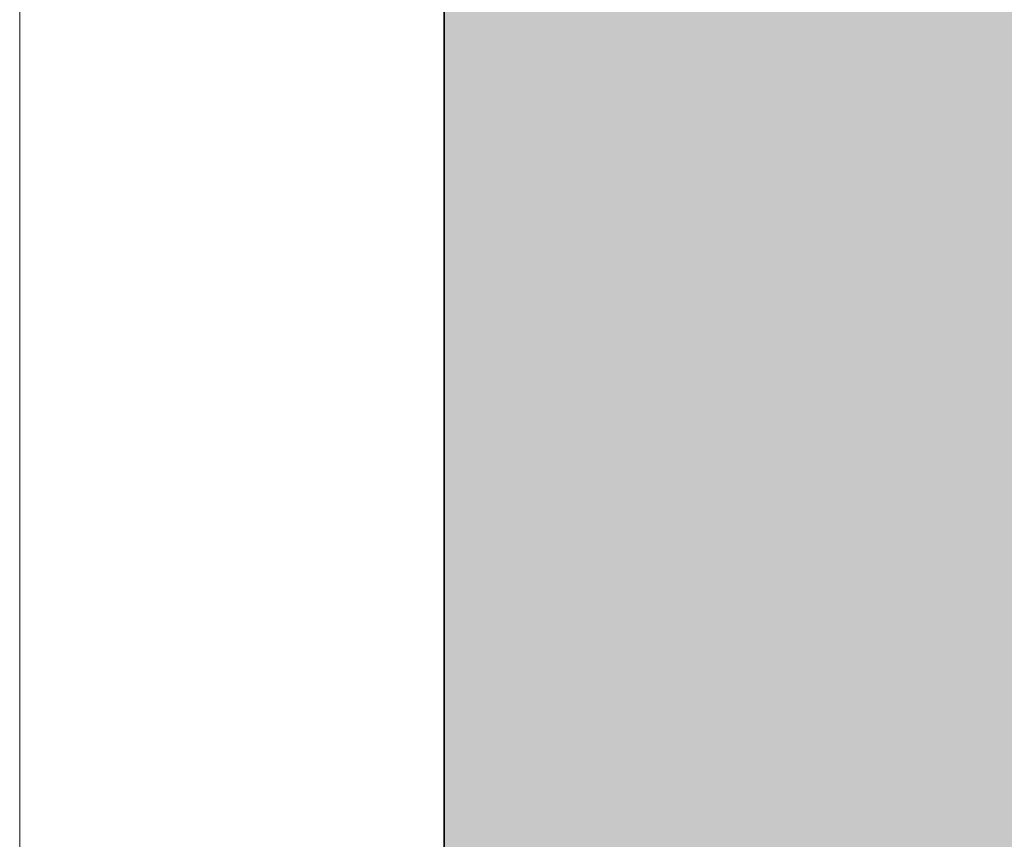
# Model space of a CAD drawing. Units: inches. Extents: x 2091 to 2899, y 967 to 2217.
# Tile 191 of 256: x 2203.11574 to 2203.18039, y 1152.30086 to 1152.35465. Entities that reach past the tile are written whole.
import ezdxf

# ---------------------------------------------------------------- set-up
doc = ezdxf.new("R2010")
doc.units = ezdxf.units.IN
doc.layers.add('A-GLAZ', color=4, linetype='Continuous', lineweight=18)
doc.layers.add('C-PROP', color=7, linetype='Continuous', lineweight=35)
doc.layers.add('A-WALL-PATT', color=141, linetype='Continuous', lineweight=13, true_color=0xadddf7)

# ---------------------------------------------------------------- blocks, each defined once
blk = doc.blocks.new('WIN-DOUBLE-LINE')
blk.add_line((0.000398, -0.000445), (0.000398, 80.8229))

msp = doc.modelspace()

# ---------------------------------------------------------------- hatches: boundary and pattern name
at = {"layer": 'A-WALL-PATT'}
h = msp.add_hatch(color=256, dxfattribs=at)
h.dxf.hatch_style = 1
h.paths.add_polyline_path([(2803.143603, 2050.919059), (2203.143603, 2050.919059), (2203.143603, 1090.919059), (2803.143603, 1090.919059)])
h.paths.add_polyline_path([(2635.79885, 1147.540465), (2674.524052, 1147.540465, 0.376086), (2678.529665, 1152.880202), (2678.529665, 1159.556473, 0.333335), (2674.524319, 1163.561846), (2674.524319, 1163.56185), (2674.524319, 1192.93439), (2635.805971, 1192.93439), (2597.087622, 1192.93439), (2597.087622, 1163.561846, 0.333335), (2593.082276, 1159.556473), (2593.082276, 1152.880202, 0.376086), (2597.087889, 1147.540465)], flags=0)
h.paths.add_polyline_path([(2436.010433, 1278.240778, 0.000483), (2435.952643, 1278.215027, -0.001328), (2435.935625, 1278.111693, -0.001711), (2436.11644, 1278.040758, 0.002185)], flags=0)
h.paths.add_polyline_path([(2794.143603, 1143.419059), (2794.143603, 1347.419059), (2543.370171, 1347.419059), (2543.370171, 1351.919059), (2794.143603, 1351.919059), (2794.143603, 1392.713555), (2793.947398, 1392.713555), (2793.947398, 1473.5369), (2794.143603, 1473.5369), (2794.143603, 1531.919059), (2650.143603, 1531.919059), (2650.143603, 1536.419059), (2794.143603, 1536.419059), (2794.143603, 1692.419059), (2609.375609, 1692.419059), (2609.375609, 1644.419059), (2604.875609, 1644.419059), (2604.875609, 1744.919059), (2609.375609, 1744.919059), (2609.375609, 1696.919059), (2794.143603, 1696.919059), (2794.143603, 1780.919059), (2609.643603, 1780.919059), (2493.875609, 1780.919059), (2493.875609, 1785.419059), (2609.643603, 1785.419059), (2794.143603, 1785.419059), (2794.143603, 1847.938821), (2793.951222, 1847.938821), (2793.951222, 1928.762166), (2794.143603, 1928.762166), (2794.143603, 1941.419059), (2614.143603, 1941.419059), (2614.143603, 1821.419059), (2609.643603, 1821.419059), (2609.643603, 1941.419059), (2392.143603, 1941.419059), (2392.143603, 1819.919059), (2387.643603, 1819.919059), (2387.643603, 1941.419059), (2212.143603, 1941.419059), (2212.143603, 1783.919059), (2392.143603, 1783.919059), (2392.143603, 1780.919059), (2212.143603, 1780.919059), (2212.143603, 1629.419059), (2387.643603, 1629.419059), (2387.643603, 1744.919059), (2392.143603, 1744.919059), (2392.143603, 1627.919059), (2317.143603, 1627.919059), (2317.143603, 1551.419059), (2317.143603, 1536.419059), (2459.383591, 1536.419059), (2459.383591, 1602.39648), (2463.883591, 1602.39648), (2463.883591, 1531.919059), (2456.643603, 1531.919059), (2456.643603, 1529.919059), (2452.143603, 1529.919059), (2452.143603, 1531.919059), (2312.643603, 1531.919059), (2312.643603, 1551.419059), (2306.143603, 1551.419059), (2306.143603, 1555.919059), (2308.143603, 1555.919059), (2308.143603, 1551.419059), (2312.643603, 1551.419059), (2312.643603, 1627.919059), (2212.143603, 1627.919059), (2212.143603, 1555.919059), (2270.143603, 1555.919059), (2270.143603, 1551.419059), (2212.143603, 1551.419059), (2212.143603, 1351.919059), (2272.143603, 1351.919059), (2272.143603, 1347.419059), (2212.143603, 1347.419059), (2212.143603, 1275.419059), (2308.143603, 1275.419059), (2308.143603, 1351.919059), (2452.143603, 1351.919059), (2452.143603, 1493.919059), (2456.643603, 1493.919059), (2456.643603, 1347.419059), (2312.643603, 1347.419059), (2312.643603, 1270.919059), (2212.143603, 1270.919059), (2212.143603, 1099.919059), (2281.237523, 1099.919059), (2282.871041, 1110.913803), (2282.008341, 1116.996603), (2278.557741, 1121.420403), (2268.205641, 1128.056203), (2272.087641, 1128.056203), (2273.812941, 1131.927003), (2279.420341, 1134.691903), (2285.027841, 1135.244903), (2287.615841, 1137.456803), (2288.047141, 1138.009803), (2289.341141, 1140.774703), (2291.066541, 1139.668703), (2292.360541, 1135.244903), (2295.379841, 1136.903803), (2296.242541, 1135.797903), (2297.105241, 1133.033003), (2300.124641, 1138.009803), (2303.143941, 1138.009803), (2304.437941, 1135.797903), (2303.143941, 1133.586003), (2306.594641, 1134.691903), (2307.888741, 1133.033003), (2310.908041, 1135.244903), (2313.927441, 1134.138903), (2315.62686, 1132.427102), (2308.320041, 1117.549603), (2290.203841, 1109.807903), (2288.909841, 1103.172103), (2289.272309, 1099.919059), (2434.918227, 1099.919059), (2431.593227, 1124.788059), (2429.930227, 1169.553059), (2430.927185, 1240.519694), (2435.658926, 1238.186126), (2437.135227, 1196.554059), (2438.798227, 1143.973059), (2442.678227, 1111.998059), (2446.558227, 1099.919059), (2794.143603, 1099.919059), (2794.143603, 1138.919059), (2548.032447, 1138.919059), (2548.032447, 1143.419059), (2548.032447, 1148.819059), (2546.668457, 1148.031559), (2528.685692, 1179.178622, 0.256256), (2512.032447, 1148.819059), (2512.032447, 1143.419059), (2512.032447, 1138.919059), (2507.532447, 1138.919059), (2507.532447, 1143.419059), (2507.532447, 1148.819059, 0.256256), (2490.879202, 1179.178622), (2472.896437, 1148.031559), (2471.532447, 1148.819059), (2471.532447, 1143.419059), (2467.032447, 1143.419059), (2467.032447, 1269.945786, 0.039061), (2460.909987, 1273.580059), (2467.032447, 1273.580059), (2467.032447, 1286.325364, 0.014511), (2465.216194, 1286.761905), (2467.032447, 1287.052576), (2467.032447, 1323.419059), (2471.532447, 1323.419059), (2471.532447, 1148.819059), (2489.532447, 1179.995973), (2490.896437, 1179.208473), (2490.879202, 1179.178622, -0.256256), (2507.532447, 1148.819059), (2507.532447, 1143.419059), (2512.032447, 1143.419059), (2512.032447, 1148.819059, -0.256256), (2528.685692, 1179.178622), (2528.668457, 1179.208473), (2530.032447, 1179.995973), (2548.032447, 1148.819059), (2548.032447, 1143.419059)], flags=16)
h.paths.add_polyline_path([(2607.768546, 1200.945083), (2607.768546, 1265.030625), (2597.087622, 1281.052011), (2619.784585, 1281.052011), (2627.795278, 1337.12686), (2635.79885, 1337.12686), (2643.816663, 1337.12686), (2651.827356, 1281.052011), (2674.524319, 1281.052011), (2663.843395, 1265.030625), (2663.843395, 1200.945083), (2635.805971, 1200.945083)], flags=0)
edge = h.paths.add_edge_path(flags=0)
edge.add_ellipse((13303.896215, 1272.998725), major_axis=(-10595.31304, 0.000001), ratio=0.842303870086, start_angle=0.6282372191, end_angle=0.6465540999, ccw=False)
edge.add_ellipse((2711.70045, 1156.852678), major_axis=(2.219769, 0), ratio=0.84230387, start_angle=111.535244, end_angle=180.628237, ccw=False)
edge.add_ellipse((13303.156292, 1272.998725), major_axis=(-10593.026306, 0), ratio=0.842303869544, start_angle=0.5282714718, end_angle=0.6465540971, ccw=False)
edge.add_line((2710.764596, 1175.333295), (2710.129986, 1175.333295))
edge.add_ellipse((2710.129986, 1176.579775), major_axis=(1.479846, 0), ratio=0.84230387, start_angle=180, end_angle=270, ccw=False)
edge.add_line((2708.65014, 1176.579775), (2708.65014, 1200.782914))
edge.add_ellipse((2710.129986, 1200.782914), major_axis=(1.479846, 0), ratio=0.84230387, start_angle=90, end_angle=180, ccw=False)
edge.add_line((2710.129986, 1202.029394), (2710.465075, 1202.029394))
edge.add_ellipse((13303.156292, 1272.998725), major_axis=(-10593.026306, 0), ratio=0.842303869544, start_angle=-0.0902290886, end_angle=0.3838667788, ccw=False)
edge.add_ellipse((2710.129986, 1290.927031), major_axis=(-1.479846, 0), ratio=0.84230387, start_angle=0, end_angle=90, ccw=False)
edge.add_line((2708.65014, 1290.927031), (2708.65014, 1315.13017))
edge.add_ellipse((2710.129986, 1315.13017), major_axis=(-1.479846, 0), ratio=0.84230387, start_angle=-90, end_angle=0, ccw=False)
edge.add_line((2710.129986, 1316.37665), (2710.706314, 1316.37665))
edge.add_ellipse((3238.40172, 1296.289566), major_axis=(528.234, 0), ratio=0.8423038695, start_angle=176.34957241, end_angle=177.82004969, ccw=False)
edge.add_ellipse((2775.063043, 1071.450696), major_axis=(313.307761, 0), ratio=0.8423038695, start_angle=102.12596555, end_angle=103.78052899, ccw=False)
edge.add_ellipse((2775.063043, 1078.305698), major_axis=(-305.302891, 0), ratio=0.8423038695, start_angle=-79.790461, end_angle=-77.55537271, ccw=False)
edge.add_ellipse((2695.141767, 1541.975383), major_axis=(-250.960216, 0), ratio=0.8423038695, start_angle=99.25656601, end_angle=102.55493264)
edge.add_line((2741.410326, 1334.214255), (2747.132545, 1337.378477))
edge.add_ellipse((2747.538616, 1336.857478), major_axis=(-0.739923, 0), ratio=0.8423039, start_angle=270, end_angle=307.93313, ccw=False)
edge.add_ellipse((2747.538616, 1336.857478), major_axis=(-0.739923, 0), ratio=0.8423039, start_angle=232.06687, end_angle=270, ccw=False)
edge.add_line((2747.944687, 1337.378477), (2753.666906, 1334.214255))
edge.add_ellipse((2799.935466, 1541.975383), major_axis=(250.960216, 0), ratio=0.8423038695, start_angle=257.44506736, end_angle=260.74343399)
edge.add_ellipse((2720.014189, 1078.305698), major_axis=(305.302891, 0), ratio=0.8423038695, start_angle=77.55537271, end_angle=79.790461, ccw=False)
edge.add_ellipse((2720.014189, 1071.450696), major_axis=(-313.307761, 0), ratio=0.8423038695, start_angle=256.21947101, end_angle=257.87403445, ccw=False)
edge.add_ellipse((2256.675512, 1296.289566), major_axis=(-528.234, 0), ratio=0.8423038695, start_angle=182.17995031, end_angle=183.65042759, ccw=False)
edge.add_line((2784.370918, 1316.37665), (2784.947247, 1316.37665))
edge.add_ellipse((2784.947247, 1315.13017), major_axis=(1.479846, 0), ratio=0.84230387, start_angle=0, end_angle=90, ccw=False)
edge.add_line((2786.427093, 1315.13017), (2786.427093, 1290.927031))
edge.add_ellipse((2784.947247, 1290.927031), major_axis=(1.479846, 0), ratio=0.84230387, start_angle=270, end_angle=360, ccw=False)
edge.add_ellipse((-7808.07906, 1272.998725), major_axis=(10593.026306, 0), ratio=0.842303869544, start_angle=-0.3838667788, end_angle=0.0902290886, ccw=False)
edge.add_line((2784.612157, 1202.029394), (2784.947247, 1202.029394))
edge.add_ellipse((2784.947247, 1200.782914), major_axis=(1.479846, 0), ratio=0.84230387, start_angle=0, end_angle=90, ccw=False)
edge.add_line((2786.427093, 1200.782914), (2786.427093, 1176.579775))
edge.add_ellipse((2784.947247, 1176.579775), major_axis=(-1.479846, 0), ratio=0.84230387, start_angle=90, end_angle=180, ccw=False)
edge.add_line((2784.947247, 1175.333295), (2784.312636, 1175.333295))
edge.add_ellipse((-7808.07906, 1272.998725), major_axis=(10593.026306, 0), ratio=0.842303869544, start_angle=-0.6186431963, end_angle=-0.5282714718, ccw=False)
edge.add_ellipse((2783.376783, 1156.852678), major_axis=(-2.219769, 0), ratio=0.84230387, start_angle=179.371763, end_angle=248.464757, ccw=False)
edge.add_ellipse((-7808.818983, 1272.998725), major_axis=(-10595.31304, 0.000004), ratio=0.842303865762, start_angle=179.3534459226, end_angle=179.3717628034, ccw=False)
edge.add_ellipse((2780.297303, 1153.500793), major_axis=(-5.246426, 0), ratio=0.84230387, start_angle=90, end_angle=179.353446, ccw=False)
edge.add_line((2780.297303, 1149.081708), (2714.77993, 1149.081708))
edge.add_ellipse((2714.77993, 1153.500793), major_axis=(5.246426, 0), ratio=0.84230387, start_angle=180.646554, end_angle=270, ccw=False)
edge = h.paths.add_edge_path(flags=0)
edge.add_line((2718.187367, 1151.007833), (2718.187367, 1170.472364))
edge.add_ellipse((2721.14706, 1170.472364), major_axis=(-2.959692, 0), ratio=0.84230387, start_angle=-90, end_angle=0, ccw=False)
edge.add_line((2721.14706, 1172.965324), (2773.930173, 1172.965324))
edge.add_ellipse((2773.930173, 1170.472364), major_axis=(-2.959692, 0), ratio=0.84230387, start_angle=180, end_angle=270, ccw=False)
edge.add_line((2776.889865, 1170.472364), (2776.889865, 1151.007833))
edge.add_line((2776.889865, 1151.007833), (2718.187367, 1151.007833))
edge = h.paths.add_edge_path(flags=0)
edge.add_line((2718.187367, 1180.23415), (2718.187367, 1199.057834))
edge.add_ellipse((2747.538616, 1320.39864), major_axis=(147.017924, 0), ratio=0.8423038695, start_angle=256.40186531, end_angle=283.59813469)
edge.add_line((2776.889865, 1199.057834), (2776.889865, 1180.23415))
edge.add_ellipse((2747.538616, 1301.574956), major_axis=(147.017924, 0), ratio=0.8423038695, start_angle=256.40186531, end_angle=283.59813469, ccw=False)
edge = h.paths.add_edge_path(flags=0)
edge.add_ellipse((13303.156292, 1272.998725), major_axis=(-10591.54646, 0), ratio=0.842303869555, start_angle=0.0555943135, end_angle=0.3777641939, ccw=False)
edge.add_line((2711.616859, 1262.72171), (2715.667408, 1249.495396))
edge.add_ellipse((6413.891963, 1241.691919), major_axis=(-3698.236159, 0), ratio=0.84230386955, start_angle=-0.120897369, end_angle=0.364076349)
edge.add_line((2715.761038, 1218.192455), (2711.934307, 1203.167361))
edge = h.paths.add_edge_path(flags=0)
edge.add_line((2718.187367, 1251.074566), (2716.002485, 1267.450435))
edge.add_ellipse((2742.151175, 1202.18954), major_axis=(81.772585, 0), ratio=0.84230387, start_angle=94.27742096, end_angle=111.8349538, ccw=False)
edge.add_line((2737.009748, 1270.930626), (2758.067484, 1270.930626))
edge.add_ellipse((2752.926058, 1202.18954), major_axis=(81.772585, 0), ratio=0.84230387, start_angle=68.1650462, end_angle=85.72257904, ccw=False)
edge.add_line((2779.074747, 1267.450435), (2776.889865, 1251.074566))
edge.add_ellipse((2750.338059, 1187.885356), major_axis=(79.579664, 0), ratio=0.84230387, start_angle=67.20808512, end_angle=85.1299304)
edge.add_line((2756.034656, 1254.743656), (2739.042576, 1254.743656))
edge.add_ellipse((2744.739174, 1187.885356), major_axis=(79.579664, 0), ratio=0.84230387, start_angle=94.8700696, end_angle=112.79191488)
edge = h.paths.add_edge_path(flags=0)
edge.add_line((2783.142926, 1203.167361), (2779.316194, 1218.192455))
edge.add_ellipse((-918.81473, 1241.691919), major_axis=(3698.236159, 0), ratio=0.84230386955, start_angle=-0.364076349, end_angle=0.120897369)
edge.add_line((2779.409825, 1249.495396), (2783.460373, 1262.72171))
edge.add_ellipse((-7808.07906, 1272.998725), major_axis=(-10591.54646, 0), ratio=0.84230386954, start_angle=179.6222358061, end_angle=179.9444056865, ccw=False)
edge = h.paths.add_edge_path(flags=0)
edge.add_ellipse((2734.200892, 1286.69044), major_axis=(-0.356609, 6.340078), ratio=0.60383358, start_angle=89.0020143, end_angle=253.657408, ccw=False)
edge.add_line((2730.369001, 1286.541806), (2730.369001, 1301.35198))
edge.add_line((2730.369001, 1301.35198), (2735.913311, 1305.214803))
edge.add_ellipse((2736.384917, 1304.734561), major_axis=(0.739923, 0), ratio=0.8423039, start_angle=90, end_angle=134.480211, ccw=False)
edge.add_line((2736.384917, 1305.357801), (2738.032783, 1305.357801))
edge.add_line((2738.032783, 1305.357801), (2738.032783, 1307.707927))
edge.add_ellipse((2794.201642, 1307.707927), major_axis=(56.168859, 0), ratio=0.84230387, start_angle=150.5614304, end_angle=180, ccw=False)
edge.add_ellipse((2700.875591, 1307.707927), major_axis=(-56.168859, 0), ratio=0.84230387, start_angle=180, end_angle=209.4385696, ccw=False)
edge.add_line((2757.04445, 1307.707927), (2757.04445, 1305.357801))
edge.add_line((2757.04445, 1305.357801), (2758.692316, 1305.357801))
edge.add_ellipse((2758.692316, 1304.734561), major_axis=(-0.739923, 0), ratio=0.8423039, start_angle=225.519789, end_angle=270, ccw=False)
edge.add_line((2759.163922, 1305.214803), (2764.708231, 1301.35198))
edge.add_line((2764.708231, 1301.35198), (2764.708231, 1286.541806))
edge.add_ellipse((2760.87634, 1286.69044), major_axis=(0.356609, 6.340078), ratio=0.60383358, start_angle=106.342592, end_angle=270.9979857, ccw=False)
edge.add_line((2757.04445, 1285.79709), (2757.04445, 1307.707927))
edge.add_ellipse((2700.875591, 1307.707927), major_axis=(-56.168859, 0), ratio=0.84230387, start_angle=180, end_angle=209.4385696)
edge.add_ellipse((2794.201642, 1307.707927), major_axis=(56.168859, 0), ratio=0.84230387, start_angle=150.5614304, end_angle=180)
edge.add_line((2738.032783, 1307.707927), (2738.032783, 1285.79709))
h.paths.add_polyline_path([(2417.812273, 1104.449704), (2413.492273, 1102.529704), (2410.612273, 1103.969704), (2409.172273, 1106.369704), (2407.252273, 1107.329704), (2406.292273, 1109.729704), (2405.332273, 1114.049704), (2405.332273, 1117.889704), (2406.292273, 1120.129704), (2407.252273, 1119.809704), (2408.848322, 1118.327658), (2410.173945, 1119.42417), (2410.211273, 1120.405704), (2411.040731, 1121.419054), (2410.699273, 1119.858704), (2410.173945, 1119.42417), (2410.088452, 1117.176109), (2411.132836, 1116.206324), (2413.972273, 1119.329704), (2416.852273, 1120.769704), (2416.869721, 1120.798784), (2417.035071, 1119.405116), (2417.896213, 1118.143384), (2418.292273, 1118.369704), (2419.544447, 1120.039269), (2419.360915, 1118.387487), (2419.032108, 1119.356151), (2418.398939, 1118.511926), (2419.252273, 1114.529704), (2418.794091, 1107.198795)], flags=0)
h.paths.add_polyline_path([(2508.870171, 1347.419059), (2508.370171, 1347.419059), (2508.370171, 1351.919059), (2508.870171, 1351.919059)], flags=0)
h.paths.add_polyline_path([(2473.370171, 1347.419059), (2472.370171, 1347.419059), (2467.870171, 1347.419059), (2467.870171, 1455.419059), (2472.370171, 1455.419059), (2472.370171, 1352.419059), (2473.370171, 1352.419059)], flags=0)
h.paths.add_polyline_path([(2352.106244, 1217.446197), (2349.226244, 1218.886197), (2347.786244, 1221.286197), (2345.866244, 1222.246197), (2344.906244, 1224.646197), (2343.946244, 1228.966197), (2343.946244, 1232.806197), (2344.906244, 1235.046197), (2345.866244, 1234.726197), (2347.462293, 1233.244152), (2348.787916, 1234.340663), (2348.825244, 1235.322197), (2349.654702, 1236.335547), (2349.313244, 1234.775197), (2348.787916, 1234.340663), (2348.702423, 1232.092603), (2349.746807, 1231.122817), (2352.586244, 1234.246197), (2355.466244, 1235.686197), (2355.483692, 1235.715277), (2355.649043, 1234.321609), (2356.510185, 1233.059877), (2356.906244, 1233.286197), (2358.158418, 1234.955762), (2357.974887, 1233.30398), (2357.646079, 1234.272644), (2357.012911, 1233.428419), (2357.866244, 1229.446197), (2357.408062, 1222.115288), (2356.426244, 1219.366197)], flags=0)
h.paths.add_polyline_path([(2348.2968, 1112.22442), (2347.0138, 1112.31042), (2345.5298, 1114.12742), (2345.7318, 1115.85842), (2346.8118, 1116.98242), (2346.8118, 1114.64642), (2345.8668, 1114.21442), (2346.8798, 1114.30042)], flags=0)
h.paths.add_polyline_path([(2347.0138, 1110.92642), (2346.2718, 1110.49342), (2346.6098, 1111.18642)], flags=0)
h.paths.add_polyline_path([(2345.8668, 1118.19442), (2345.5298, 1117.32942), (2343.7078, 1118.02142), (2344.3828, 1118.62642)], flags=0)
h.paths.add_polyline_path([(2346.6768, 1109.28242), (2346.0698, 1108.07142), (2345.8668, 1110.06142)], flags=0)
h.paths.add_polyline_path([(2345.0568, 1119.75142), (2343.6398, 1119.75142), (2343.9778, 1121.13542)], flags=0)
h.paths.add_polyline_path([(2345.2598, 1116.55042), (2345.1248, 1115.85842), (2344.9218, 1115.68542), (2344.7198, 1116.37742)], flags=0)
h.paths.add_polyline_path([(2345.6648, 1112.31042), (2345.4618, 1111.53242), (2344.0448, 1111.96442), (2344.6518, 1112.57042)], flags=0)
h.paths.add_polyline_path([(2345.1918, 1113.34942), (2344.4498, 1113.86842), (2344.7198, 1114.38742)], flags=0)
h.paths.add_polyline_path([(2344.6518, 1116.80942), (2344.1798, 1115.68542), (2344.6518, 1115.33942), (2343.9098, 1114.90642), (2343.0328, 1115.94442), (2343.6398, 1116.46342)], flags=0)
h.paths.add_polyline_path([(2345.8668, 1106.68642), (2344.9898, 1105.56242), (2344.5168, 1106.60042)], flags=0)
h.paths.add_polyline_path([(2344.8548, 1110.06142), (2344.5168, 1109.28242), (2344.1128, 1109.71542)], flags=0)
h.paths.add_polyline_path([(2344.0448, 1113.52242), (2343.4378, 1113.08942), (2342.7628, 1113.95442)], flags=0)
h.paths.add_polyline_path([(2344.3148, 1111.01242), (2342.9648, 1110.32042), (2342.9648, 1111.09942)], flags=0)
h.paths.add_polyline_path([(2345.1248, 1104.69742), (2344.5848, 1103.74542), (2344.4498, 1104.26442)], flags=0)
h.paths.add_polyline_path([(2342.8298, 1121.22242), (2341.7498, 1120.53042), (2340.5358, 1121.04942), (2340.1308, 1121.82842), (2340.6708, 1122.95242), (2341.1428, 1121.82842), (2341.6148, 1122.00142)], flags=0)
h.paths.add_polyline_path([(2342.9648, 1119.75142), (2343.0328, 1118.45342), (2342.0878, 1118.02142), (2342.0198, 1119.49142)], flags=0)
h.paths.add_polyline_path([(2342.6948, 1116.89642), (2341.9528, 1116.63642), (2342.0198, 1117.32942)], flags=0)
h.paths.add_polyline_path([(2343.0328, 1112.22442), (2342.0198, 1111.79142), (2341.5478, 1112.22442), (2342.3578, 1113.34942)], flags=0)
h.paths.add_polyline_path([(2343.7748, 1104.43742), (2342.6278, 1102.88042), (2342.6948, 1104.61042), (2343.4378, 1105.12942)], flags=0)
h.paths.add_polyline_path([(2342.0198, 1115.07942), (2340.8058, 1115.51242), (2340.9408, 1116.37742)], flags=0)
h.paths.add_polyline_path([(2341.4808, 1120.09742), (2341.4808, 1119.40542), (2341.0758, 1119.57842), (2341.1428, 1120.09742)], flags=0)
h.paths.add_polyline_path([(2341.8178, 1114.47342), (2340.9408, 1113.08942), (2340.8058, 1114.56042)], flags=0)
h.paths.add_polyline_path([(2341.1428, 1118.54042), (2340.9408, 1116.98242), (2339.0508, 1117.67542), (2339.0508, 1118.62642)], flags=0)
h.paths.add_polyline_path([(2342.6948, 1101.66842), (2341.9528, 1101.84142), (2342.5598, 1102.36142)], flags=0)
h.paths.add_polyline_path([(2340.3328, 1119.66542), (2338.4438, 1119.57842), (2337.9038, 1120.35742), (2339.6578, 1120.61642)], flags=0)
h.paths.add_polyline_path([(2340.3328, 1115.33942), (2340.0628, 1113.69542), (2339.3878, 1115.33942)], flags=0)
h.paths.add_polyline_path([(2341.8178, 1103.83142), (2341.5478, 1102.88042), (2341.1428, 1103.65842)], flags=0)
h.paths.add_polyline_path([(2339.0508, 1122.86642), (2337.2958, 1121.82842), (2337.0938, 1123.12542), (2337.7688, 1123.81842)], flags=0)
h.paths.add_polyline_path([(2339.1178, 1121.74142), (2338.8478, 1121.22242), (2338.1738, 1121.04942), (2338.3758, 1121.56842)], flags=0)
h.paths.add_polyline_path([(2339.1858, 1119.31942), (2338.6458, 1118.71342), (2338.2408, 1118.10742), (2338.2408, 1118.88642)], flags=0)
h.paths.add_polyline_path([(2341.1428, 1101.92842), (2340.6028, 1101.23642), (2340.0628, 1101.84142), (2340.6028, 1102.36142)], flags=0)
h.paths.add_polyline_path([(2337.6338, 1117.76142), (2336.6208, 1118.28042), (2337.2958, 1118.97242)], flags=0)
h.paths.add_polyline_path([(2336.8238, 1119.57842), (2334.7988, 1118.97242), (2335.2038, 1120.35742), (2336.5538, 1120.87642)], flags=0)
h.paths.add_polyline_path([(2339.1178, 1100.45742), (2337.3638, 1100.54342), (2336.7558, 1101.23642)], flags=0)
h.paths.add_polyline_path([(2336.3508, 1122.43342), (2336.0138, 1121.91442), (2334.9338, 1122.43342), (2334.5288, 1123.47142), (2335.7438, 1122.77942)], flags=0)
h.paths.add_polyline_path([(2334.7318, 1120.87642), (2334.2588, 1120.35742), (2334.0568, 1120.78942), (2334.5968, 1121.30842)], flags=0)
h.paths.add_polyline_path([(2334.4618, 1122.17442), (2332.5718, 1121.30842), (2331.3568, 1122.17442), (2332.0998, 1122.86642)], flags=0)
h.paths.add_polyline_path([(2334.2588, 1118.54042), (2333.3818, 1118.45342), (2333.6518, 1119.31942)], flags=0)
h.paths.add_polyline_path([(2335.5418, 1102.27442), (2334.1918, 1102.62042), (2335.2718, 1103.31242)], flags=0)
h.paths.add_polyline_path([(2332.7068, 1119.66542), (2331.6948, 1120.44342), (2332.5048, 1120.78942)], flags=0)
h.paths.add_polyline_path([(2334.7318, 1101.14942), (2333.5168, 1101.58242), (2333.9888, 1101.75542)], flags=0)
h.paths.add_polyline_path([(2332.6398, 1116.63642), (2331.0868, 1116.29042), (2331.9648, 1118.19442)], flags=0)
h.paths.add_polyline_path([(2330.7498, 1121.56842), (2330.2768, 1120.27042), (2328.5228, 1119.31942), (2328.9948, 1121.04942)], flags=0)
h.paths.add_polyline_path([(2330.7498, 1118.62642), (2330.0078, 1117.50242), (2329.8728, 1118.02142)], flags=0)
h.paths.add_polyline_path([(2332.0998, 1102.36142), (2330.5468, 1102.01442), (2331.6948, 1102.96642)], flags=0)
h.paths.add_polyline_path([(2329.5348, 1113.60842), (2329.0628, 1112.31042), (2328.5898, 1113.34942)], flags=0)
h.paths.add_polyline_path([(2328.3878, 1117.84842), (2327.5098, 1116.55042), (2327.1728, 1117.76142)], flags=0)
h.paths.add_polyline_path([(2329.7378, 1106.51342), (2329.5348, 1105.30242), (2328.2528, 1106.08142)], flags=0)
h.paths.add_polyline_path([(2328.6578, 1114.38742), (2328.0498, 1114.12742), (2328.3198, 1114.90642)], flags=0)
h.paths.add_polyline_path([(2328.3198, 1112.22442), (2327.1058, 1112.13742), (2326.7008, 1112.65642)], flags=0)
h.paths.add_polyline_path([(2326.9028, 1115.25242), (2326.7008, 1114.12742), (2325.2158, 1113.60842), (2326.0928, 1115.33942)], flags=0)
h.paths.add_polyline_path([(2326.6328, 1108.33042), (2326.0928, 1107.37942), (2325.8908, 1108.50342), (2326.4978, 1109.10942)], flags=0)
h.paths.add_polyline_path([(2615.143603, 1531.919059), (2609.643603, 1531.919059), (2609.643603, 1620.419059), (2614.143603, 1620.419059), (2614.143603, 1536.419059), (2615.143603, 1536.419059)], flags=0)
h.paths.add_polyline_path([(2545.143603, 1563.419059), (2464.143603, 1563.419059), (2464.143603, 1632.419059), (2509.143603, 1632.419059), (2509.143603, 1627.919059), (2509.143603, 1603.919059), (2468.643603, 1603.919059), (2468.643603, 1567.919059), (2540.643603, 1567.919059), (2540.643603, 1591.919059), (2545.143603, 1591.919059)], flags=0)
h.paths.add_polyline_path([(2388.969048, 1549.985735), (2357.434181, 1549.985735), (2357.434181, 1623.360778), (2399.362777, 1623.360778), (2435.689465, 1623.360778), (2435.592547, 1602.559273), (2435.592547, 1602.39648), (2388.969048, 1602.39648)], flags=0)
h.paths.add_polyline_path([(2388.880628, 1555.809151), (2374.904429, 1555.809151), (2374.904429, 1600.571564), (2374.904429, 1615.457645), (2406.350877, 1615.457645), (2406.350877, 1618.939431), (2412.174293, 1615.457645), (2406.350877, 1611.97586), (2406.350877, 1615.457645), (2388.880628, 1615.457645)], flags=0)
h.paths.add_polyline_path([(2568.875609, 1644.419059), (2453.375609, 1644.419059), (2453.375609, 1785.419059), (2457.875609, 1785.419059), (2457.875609, 1648.919059), (2568.875609, 1648.919059)], flags=0)
h.paths.add_polyline_path([(2212.143603, 1945.919059), (2212.143603, 2041.919059), (2794.143603, 2041.919059), (2794.143603, 1945.919059)], flags=16)
h.paths.add_polyline_path([(2271.082728, 1964.317238), (2776.852968, 1964.317238), (2776.852968, 2037.169623), (2271.082728, 2037.169623)], flags=8)
h.paths.add_polyline_path([(2380.649285, 1536.824144), (2461.040809, 1536.824144), (2461.040809, 1554.652587), (2380.649285, 1554.652587)], flags=8)
h.paths.add_polyline_path([(2240.755709, 1609.725451), (2309.185829, 1609.725451), (2309.185829, 1617.698204), (2240.755709, 1617.698204)], flags=8)
h.paths.add_polyline_path([(2212.677255, 1313.504102), (2282.59152, 1313.504102), (2282.59152, 1322.745239), (2212.677255, 1322.745239)], flags=8)
h.paths.add_polyline_path([(2457.111976, 1114.778574), (2558.481581, 1114.778574), (2558.481581, 1142.219682), (2457.111976, 1142.219682)], flags=8)
h.paths.add_polyline_path([(2473.442337, 1273.010067), (2604.641226, 1273.010067), (2604.641226, 1318.346935), (2473.442337, 1318.346935)], flags=8)
h.paths.add_polyline_path([(2638.876302, 1626.977432), (2684.250367, 1627.976738), (2684.038483, 1637.597494), (2638.664417, 1636.598188)], flags=8)
h.paths.add_polyline_path([(2537.590554, 1453.793447), (2628.389547, 1453.793447), (2628.389547, 1475.344811), (2537.590554, 1475.344811)], flags=8)
h.paths.add_polyline_path([(2504.137638, 1714.632397), (2554.647187, 1714.632397), (2554.647187, 1730.237712), (2504.137638, 1730.237712)], flags=8)
h.paths.add_polyline_path([(2487.501181, 1575.651872), (2535.097121, 1575.651872), (2535.097121, 1598.377646), (2487.501181, 1598.377646)], flags=8)
h.paths.add_polyline_path([(2709.0994, 1735.710278), (2740.016601, 1735.710278), (2740.016601, 1749.937641), (2709.0994, 1749.937641)], flags=8)
h.paths.add_polyline_path([(2442.438424, 1792.171657), (2564.728835, 1792.171657), (2564.728835, 1842.000163), (2442.438424, 1842.000163)], flags=8)
h.paths.add_polyline_path([(2655.815801, 1809.644076), (2789.520142, 1806.693796), (2790.084977, 1832.291638), (2656.380635, 1835.241918)], flags=8)
h.paths.add_polyline_path([(2234.842697, 1797.720143), (2368.592851, 1794.768852), (2369.160718, 1820.504132), (2235.410564, 1823.455423)], flags=8)
h.paths.add_polyline_path([(2245.138466, 1644.006335), (2398.427733, 1640.6239), (2398.994842, 1666.32482), (2245.705575, 1669.707255)], flags=8)
h.paths.add_polyline_path([(2306.142847, 1431.168519), (2413.768314, 1428.793687), (2414.333148, 1454.391529), (2306.707682, 1456.76636)], flags=8)
h.paths.add_polyline_path([(2306.834582, 1458.233145), (2393.380484, 1456.323449), (2393.932808, 1481.354358), (2307.386907, 1483.264054)], flags=8)

# ---------------------------------------------------------------- linework, layer by layer
at = {"layer": 'C-PROP'}
msp.add_lwpolyline([(2203.143603, 2050.919059), (2803.143603, 2050.919059), (2803.143603, 1090.919059), (2203.143603, 1090.919059)], close=True, dxfattribs=at)

# ---------------------------------------------------------------- block references
at = {"layer": 'A-GLAZ'}
msp.add_blockref('WIN-DOUBLE-LINE', (2203.115344, 1152.247505), dxfattribs=at)

doc.saveas('drawing.dxf')
